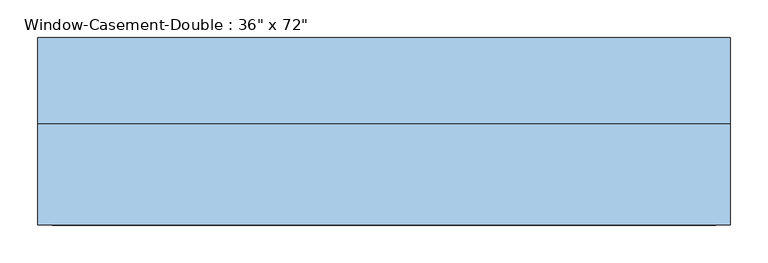
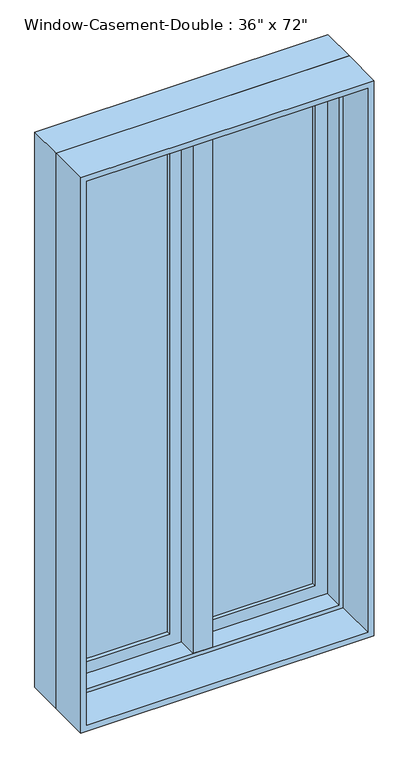
"""IFC4 building model written with IfcOpenShell, lengths in millimetres: window geometry."""

from ifc_helpers import new_model, si_unit, frame, origin, place, context, project, spatial, polyline, outline, extrude, faceted_brep, source, transform, mapped, element, save


def window_5590b26e(model_context):
    return source(origin(), model_context, "Body", "SolidModel", [
        faceted_brep([(9.525, 133.35, 2730.5), (-9.525, 133.35, 2730.5), (-9.525, 82.55, 2730.5), (9.525, 82.55, 2730.5), (9.525, 133.35, 927.1), (9.525, 82.55, 927.1), (-9.525, 82.55, 927.1), (-9.525, 133.35, 927.1), (-9.525, 82.55, 946.15), (-9.525, 82.55, 2711.45), (-30.1625, 82.55, 946.15), (-30.1625, 82.55, 2711.45), (-30.1625, 19.05, 946.15), (-30.1625, 19.05, 2711.45), (30.1625, 19.05, 946.15), (30.1625, 19.05, 2711.45), (30.1625, 82.55, 946.15), (30.1625, 82.55, 2711.45), (9.525, 82.55, 946.15), (9.525, 82.55, 2711.45)], [[[0, 1, 2, 3]], [[4, 5, 6, 7]], [[1, 0, 4, 7]], [[2, 1, 7, 6, 8, 9]], [[9, 8, 10, 11]], [[11, 10, 12, 13]], [[13, 12, 14, 15]], [[15, 14, 16, 17]], [[17, 16, 18, 19]], [[0, 3, 19, 18, 5, 4]], [[18, 8, 6, 5]], [[9, 19, 3, 2]], [[8, 18, 16, 14, 12, 10]], [[19, 9, 11, 13, 15, 17]]]),
        extrude(outline(polyline([(-66.675, 114.3), (-66.675, 107.95), (-387.35, 107.95), (-387.35, 114.3), (-66.675, 114.3)])), frame((0.0, 0.0, 984.25), z_axis=(0.0, 0.0, 1.0), x_axis=(1.0, 0.0, 0.0)), (0.0, 0.0, 1.0), 1689.1),
        extrude(outline(polyline([(-387.35, 95.25), (-387.35, 101.6), (-66.675, 101.6), (-66.675, 95.25), (-387.35, 95.25)])), frame((0.0, 0.0, 984.25), z_axis=(0.0, 0.0, 1.0), x_axis=(1.0, 0.0, 0.0)), (0.0, 0.0, 1.0), 1689.1),
        extrude(outline(polyline([(387.35, 114.3), (387.35, 107.95), (66.675, 107.95), (66.675, 114.3), (387.35, 114.3)])), frame((0.0, 0.0, 984.25), z_axis=(0.0, 0.0, 1.0), x_axis=(1.0, 0.0, 0.0)), (0.0, 0.0, 1.0), 1689.1),
        extrude(outline(polyline([(66.675, 95.25), (66.675, 101.6), (387.35, 101.6), (387.35, 95.25), (66.675, 95.25)])), frame((0.0, 0.0, 984.25), z_axis=(0.0, 0.0, 1.0), x_axis=(1.0, 0.0, 0.0)), (0.0, 0.0, 1.0), 1689.1),
        extrude(outline(polyline([(2730.5, -444.5), (927.1, -444.5), (927.1, -9.525), (2730.5, -9.525), (2730.5, -444.5)]), holes=[polyline([(2673.35, -66.675), (984.25, -66.675), (984.25, -387.35), (2673.35, -387.35), (2673.35, -66.675)])]), frame((0.0, 82.55, 0.0), z_axis=(0.0, 1.0, 0.0), x_axis=(0.0, 0.0, 1.0)), (0.0, 0.0, 1.0), 44.45),
        extrude(outline(polyline([(927.1, 444.5), (2730.5, 444.5), (2730.5, 9.525), (927.1, 9.525), (927.1, 444.5)]), holes=[polyline([(984.25, 66.675), (2673.35, 66.675), (2673.35, 387.35), (984.25, 387.35), (984.25, 66.675)])]), frame((0.0, 82.55, 0.0), z_axis=(0.0, 1.0, 0.0), x_axis=(0.0, 0.0, 1.0)), (0.0, 0.0, 1.0), 44.45),
        extrude(outline(polyline([(2743.2, -457.2), (914.4, -457.2), (914.4, 457.2), (2743.2, 457.2), (2743.2, -457.2)]), holes=[polyline([(2724.15, 438.15), (933.45, 438.15), (933.45, -438.15), (2724.15, -438.15), (2724.15, 438.15)])]), frame((0.0, -114.3, 0.0), z_axis=(0.0, 1.0, 0.0), x_axis=(0.0, 0.0, 1.0)), (0.0, 0.0, 1.0), 133.35),
        faceted_brep([(425.45, 82.55, 2711.45), (425.45, 19.05, 2711.45), (-425.45, 19.05, 2711.45), (-425.45, 82.55, 2711.45), (444.5, 133.35, 2730.5), (444.5, 82.55, 2730.5), (-444.5, 82.55, 2730.5), (-444.5, 133.35, 2730.5), (457.2, 19.05, 2743.2), (457.2, 133.35, 2743.2), (-457.2, 133.35, 2743.2), (-457.2, 19.05, 2743.2), (-425.45, 19.05, 946.15), (-425.45, 82.55, 946.15), (-444.5, 82.55, 927.1), (-444.5, 133.35, 927.1), (-457.2, 133.35, 914.4), (-457.2, 19.05, 914.4), (425.45, 19.05, 946.15), (425.45, 82.55, 946.15), (444.5, 82.55, 927.1), (444.5, 133.35, 927.1), (457.2, 133.35, 914.4), (457.2, 19.05, 914.4)], [[[0, 1, 2, 3]], [[4, 5, 6, 7]], [[8, 9, 10, 11]], [[3, 2, 12, 13]], [[7, 6, 14, 15]], [[11, 10, 16, 17]], [[13, 12, 18, 19]], [[15, 14, 20, 21]], [[17, 16, 22, 23]], [[11, 17, 23, 8], [1, 18, 12, 2]], [[19, 18, 1, 0]], [[5, 20, 14, 6], [3, 13, 19, 0]], [[21, 20, 5, 4]], [[23, 22, 9, 8]], [[9, 22, 16, 10], [7, 15, 21, 4]]]),
    ])


if __name__ == "__main__":
    model = new_model("IFC4")
    model_context = context("Model", 3, world=origin())
    ifc_project = project(units=[si_unit("LENGTHUNIT", "METRE", prefix="MILLI")], contexts=[model_context])
    site = spatial("IfcSite", under=ifc_project)
    building = spatial("IfcBuilding", under=site)
    placement = place(None, origin())
    window_shape = window_5590b26e(model_context)
    element("IfcWindow", 1, ObjectType="Window-Casement-Double : 36\" x 72\"", at=placement, inside=building, context=model_context, shape_type="MappedRepresentation", body=[
        mapped(window_shape, transform((0.0, 0.0, 0.0), x_axis=(1.0, 0.0, 0.0), y_axis=(0.0, 1.0, 0.0), z_axis=(0.0, 0.0, 1.0))),
    ])
    save(model, "model.ifc")

# Revit data of these elements
# Type "Window-Casement-Double : 36\" x 72\""
#   Type Mark = "20"
#   Fire Rating = "0.5h"
#   Assembly Code = "B2020100"
#   Analytic Construction = "Double glazing - domestic"
#   Frame Extension [instance default] = 0' - 0 1/4"
#   Window Inset [instance default] = 0' - 0"
#   Wall Thickness [instance default] = 0' - 6"
#   Interior Wall Closure [instance default] = 0' - 2 1/4"
#   Half Width = 1' - 6"
#   Visual Light Transmittance = 0.81
#   Thermal Resistance (R) = 1.8146 (h·ft²·°F)/BTU
#   Solar Heat Gain Coefficient = 0.76
#   Rough Width = 3' - 0 1/2"
#   Rough Height = 6' - 0 1/2"
#   Height = 6' - 0"
#   Heat Transfer Coefficient (U) = 0.5511 BTU/(h·ft²·°F)
#   Exterior Wall Closure [instance default] = 0' - 1 1/4"
#   Extension Jamb [instance default] = 0' - 2 1/4"
#   Default Sill Height = 3' - 0"
#   Width = 3' - 0"
#   Muntin Visibility = yes
#   Interior Trim Visibility [instance default] = yes
#   Exterior Trim Visibility [instance default] = yes
#   Extension Jamb Visibility [instance default] = yes
#   Interior Trim Material = Wood - Stained
#   Muntin Pattern = Muntin Pattern_2x2 : Muntin Pattern_2x2
#   Interior Trim = Trim-Window-Interior-Flat : Picture Frame
#   Interior Frame Material = Wood - Stained
#   Glass Panel Material = Glass
#   Exterior Trim Material = Clad - White
#   Exterior Trim = Trim-Window-Exterior-Flat : with Sill
#   Exterior Frame Material = Clad - White
#   Wall Closure = (empty or 0)
# Element 1 (IfcWindow, "Window-Casement-Double : 36\" x 72\"")
#   Wall Thickness = 0' - 9"
#   Extension Jamb = 0' - 5 1/4"
#   Materials on its faces: "Wood - Stained", "Glass", "Clad - White"
# Materials
#   "Wood - Stained": class "Wood", colour RGB 224 178 126, transparency 0, Cost = 0
#   "Glass": class "Glass", colour RGB 0 128 192, transparency 0.75, Description = "Soda Lime Glass", Cost = 0
#   "Clad - White": class "Wood", colour RGB 242 242 238, transparency 0, Cost = 0
